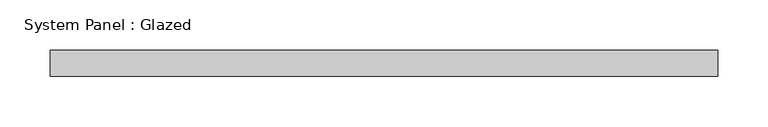
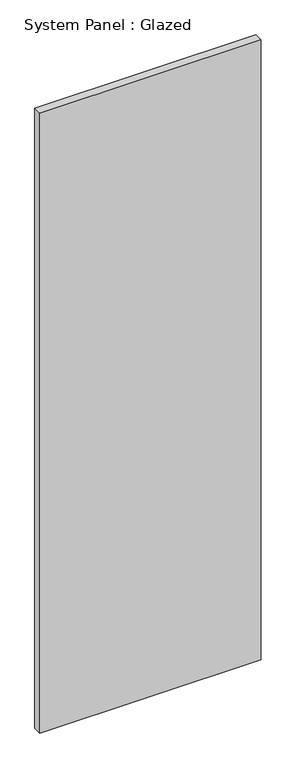
"""IFC4 building model written with IfcOpenShell, lengths in millimetres: plate geometry, System Panel : Glazed."""

from ifc_helpers import new_model, si_unit, origin, origin_with_axes, place, context, project, spatial, polyline, outline, extrude, source, transform, mapped, element, save


def system_panel_glazed_df754354(model_context):
    return source(origin(), model_context, "Body", "SweptSolid", [
        extrude(outline(polyline([(330.2, 19.05), (-330.2, 19.05), (-330.2, 44.45), (330.2, 44.45), (330.2, 19.05)])), origin_with_axes(), (0.0, 0.0, 1.0), 1953.6846597),
    ])


if __name__ == "__main__":
    model = new_model("IFC4")
    model_context = context("Model", 3, world=origin())
    ifc_project = project(units=[si_unit("LENGTHUNIT", "METRE", prefix="MILLI")], contexts=[model_context])
    site = spatial("IfcSite", under=ifc_project)
    building = spatial("IfcBuilding", under=site)
    placement = place(None, origin())
    system_panel_glazed_shape = system_panel_glazed_df754354(model_context)
    element("IfcPlate", 1, ObjectType="System Panel : Glazed", at=placement, inside=building, context=model_context, shape_type="MappedRepresentation", body=[
        mapped(system_panel_glazed_shape, transform((0.0, 0.0, 0.0), x_axis=(1.0, 0.0, 0.0), y_axis=(0.0, 1.0, 0.0), z_axis=(0.0, 0.0, 1.0))),
    ])
    save(model, "model.ifc")

# Revit data of these elements
# Type "System Panel : Glazed"
#   Construction Type Id = "GSP4R"
#   Analytic Construction = "1/8 in Pilkington single glazing"
#   Visual Light Transmittance = 0.9
#   Solar Heat Gain Coefficient = 0.86
#   Heat Transfer Coefficient (U) = 1.18115 BTU/(h·ft²·°F)
#   Define Thermal Properties by = 1
# Element 1 (IfcPlate, "System Panel : Glazed")
#   Materials on its faces: "Glass"
# Materials
#   "Glass": class "Glass", colour RGB 0 128 192, transparency 0.75, Description = "Soda Lime Glass", Cost = 0
